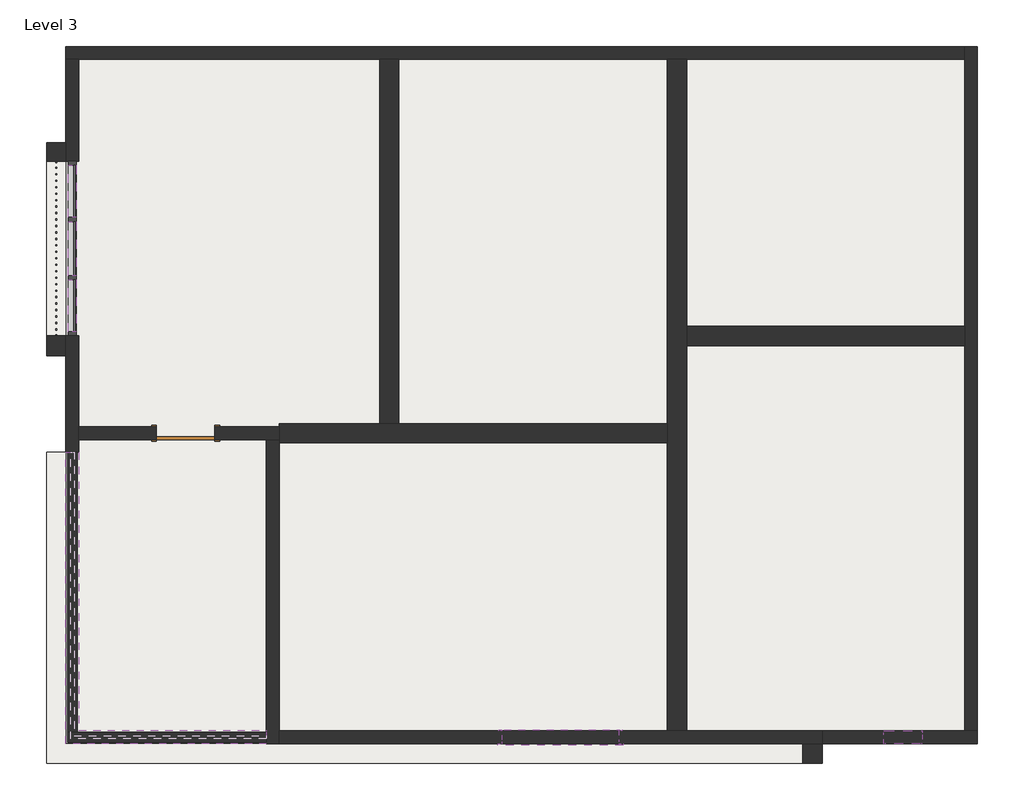
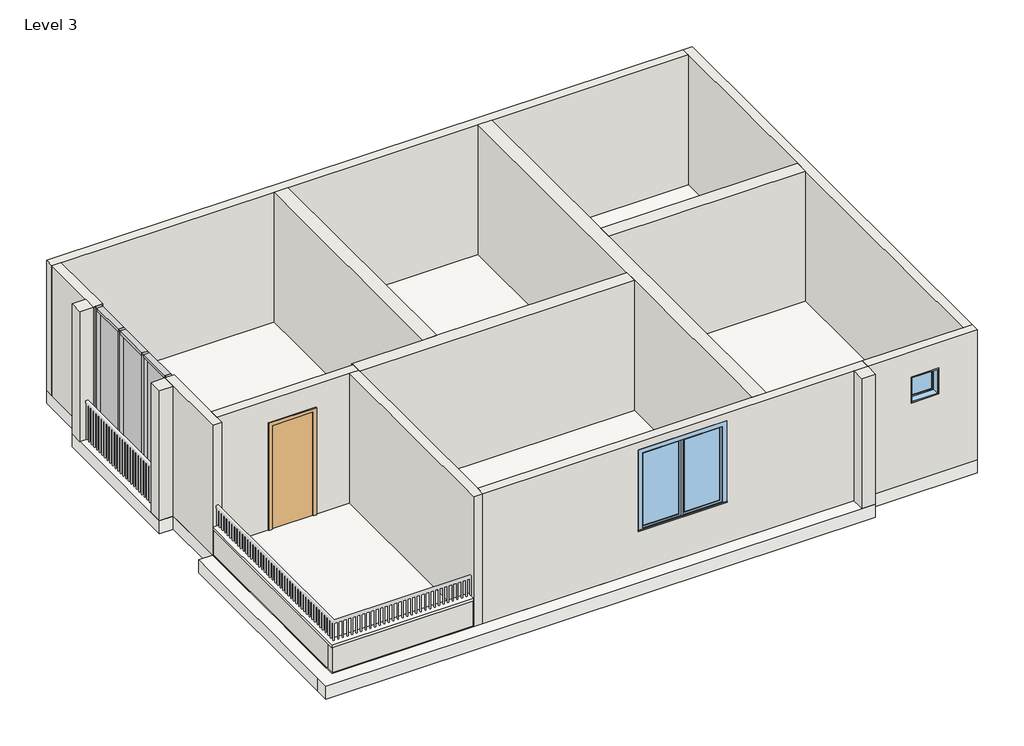
# One storey, part 1 of 2: 17 walls, 10 members, 3 plates, 3 slabs, 2 windows, 1 door.
"""IFC4 building model written with IfcOpenShell, lengths in millimetres."""

from ifc_helpers import new_model, si_unit, frame, origin, place, context, project, spatial, polyline, outline, extrude, faceted_brep, transform, mapped, element, save
from components import door_f936a269, member_eaba9652, member_3f395ae9, member_c17f1be2, member_d2e7e466, system_panel_glazed_52d31088, system_panel_glazed_f0722de2, window_97c6202a, window_6846e476

model = new_model("IFC4")

# Units and contexts
model_context = context("Model", 3, world=origin())
ifc_project = project(units=[si_unit("LENGTHUNIT", "METRE", prefix="MILLI")], contexts=[model_context])

# Site, building, storey
site = spatial("IfcSite", under=ifc_project)
building = spatial("IfcBuilding", under=site)
storey = spatial("IfcBuildingStorey", under=building, Name="Level 3", Elevation=6096.0)

# Door
placement = place(None, origin())
door_shape = door_f936a269(model_context)
element("IfcDoor", 1, ObjectType="Single-Flush : 36\" x 96\"", at=placement, inside=storey, context=model_context, shape_type="MappedRepresentation", body=[
    mapped(door_shape, transform((-16449.2169582, -4610.4617616, 6705.6), x_axis=(-1.0, 0.0, 0.0), y_axis=(0.0, -1.0, 0.0), z_axis=(0.0, 0.0, 1.0))),
])

# Members
member_shape = member_eaba9652(model_context)
element("IfcMember", 2, ObjectType="Rectangular Mullion : 2.5\" x 5\" rectangular", at=placement, inside=storey, context=model_context, shape_type="MappedRepresentation", body=[
    mapped(member_shape, transform((-18227.2169582, -1251.3117616, 6705.6), x_axis=(0.0, -1.0, 0.0), y_axis=(-1.0, 0.0, 0.0), z_axis=(0.0, 0.0, -1.0))),
])
element("IfcMember", 3, ObjectType="Rectangular Mullion : 2.5\" x 5\" rectangular", at=placement, inside=storey, context=model_context, shape_type="MappedRepresentation", body=[
    mapped(member_shape, transform((-18227.2169582, -2165.7117616, 6705.6), x_axis=(0.0, -1.0, 0.0), y_axis=(-1.0, 0.0, 0.0), z_axis=(0.0, 0.0, -1.0))),
])
member_2_shape = member_3f395ae9(model_context)
element("IfcMember", 4, ObjectType="Rectangular Mullion : 2.5\" x 5\" rectangular", at=placement, inside=storey, context=model_context, shape_type="MappedRepresentation", body=[
    mapped(member_2_shape, transform((-18227.2169582, -3080.1117616, 6705.6), x_axis=(0.0, -1.0, 0.0), y_axis=(-1.0, 0.0, 0.0), z_axis=(0.0, 0.0, -1.0))),
])
element("IfcMember", 5, ObjectType="Rectangular Mullion : 2.5\" x 5\" rectangular", at=placement, inside=storey, context=model_context, shape_type="MappedRepresentation", body=[
    mapped(member_2_shape, transform((-18227.2169582, -336.9117616, 9753.6), x_axis=(0.0, 1.0, 0.0), y_axis=(-1.0, 0.0, 0.0), z_axis=(0.0, 0.0, 1.0))),
])
member_3_shape = member_c17f1be2(model_context)
element("IfcMember", 6, ObjectType="Rectangular Mullion : 2.5\" x 5\" rectangular", at=placement, inside=storey, context=model_context, shape_type="MappedRepresentation", body=[
    mapped(member_3_shape, transform((-18227.2169582, -3016.6117616, 9753.6), x_axis=(0.0, 0.0, 1.0), y_axis=(-1.0, 0.0, 0.0), z_axis=(0.0, -1.0, 0.0))),
])
element("IfcMember", 7, ObjectType="Rectangular Mullion : 2.5\" x 5\" rectangular", at=placement, inside=storey, context=model_context, shape_type="MappedRepresentation", body=[
    mapped(member_3_shape, transform((-18227.2169582, -1219.5617616, 9753.6), x_axis=(0.0, 0.0, 1.0), y_axis=(-1.0, 0.0, 0.0), z_axis=(0.0, -1.0, 0.0))),
])
element("IfcMember", 8, ObjectType="Rectangular Mullion : 2.5\" x 5\" rectangular", at=placement, inside=storey, context=model_context, shape_type="MappedRepresentation", body=[
    mapped(member_3_shape, transform((-18227.2169582, -400.4117616, 6705.6), x_axis=(0.0, 0.0, -1.0), y_axis=(-1.0, 0.0, 0.0), z_axis=(0.0, 1.0, 0.0))),
])
element("IfcMember", 9, ObjectType="Rectangular Mullion : 2.5\" x 5\" rectangular", at=placement, inside=storey, context=model_context, shape_type="MappedRepresentation", body=[
    mapped(member_3_shape, transform((-18227.2169582, -2197.4617616, 6705.6), x_axis=(0.0, 0.0, -1.0), y_axis=(-1.0, 0.0, 0.0), z_axis=(0.0, 1.0, 0.0))),
])
member_4_shape = member_d2e7e466(model_context)
element("IfcMember", 10, ObjectType="Rectangular Mullion : 2.5\" x 5\" rectangular", at=placement, inside=storey, context=model_context, shape_type="MappedRepresentation", body=[
    mapped(member_4_shape, transform((-18227.2169582, -1283.0617616, 6705.6), x_axis=(0.0, 0.0, -1.0), y_axis=(-1.0, 0.0, 0.0), z_axis=(0.0, 1.0, 0.0))),
])
element("IfcMember", 11, ObjectType="Rectangular Mullion : 2.5\" x 5\" rectangular", at=placement, inside=storey, context=model_context, shape_type="MappedRepresentation", body=[
    mapped(member_4_shape, transform((-18227.2169582, -2133.9617616, 9753.6), x_axis=(0.0, 0.0, 1.0), y_axis=(-1.0, 0.0, 0.0), z_axis=(0.0, -1.0, 0.0))),
])

# Plates
system_panel_glazed_shape = system_panel_glazed_52d31088(model_context)
element("IfcPlate", 12, ObjectType="System Panel : Glazed", at=placement, inside=storey, context=model_context, shape_type="MappedRepresentation", body=[
    mapped(system_panel_glazed_shape, transform((-18227.2169582, -809.9867616, 6769.1), x_axis=(0.0, -1.0, 0.0), y_axis=(1.0, 0.0, 0.0), z_axis=(0.0, 0.0, 1.0))),
])
element("IfcPlate", 13, ObjectType="System Panel : Glazed", at=placement, inside=storey, context=model_context, shape_type="MappedRepresentation", body=[
    mapped(system_panel_glazed_shape, transform((-18227.2169582, -2607.0367616, 6769.1), x_axis=(0.0, -1.0, 0.0), y_axis=(1.0, 0.0, 0.0), z_axis=(0.0, 0.0, 1.0))),
])
system_panel_glazed_2_shape = system_panel_glazed_f0722de2(model_context)
element("IfcPlate", 14, ObjectType="System Panel : Glazed", at=placement, inside=storey, context=model_context, shape_type="MappedRepresentation", body=[
    mapped(system_panel_glazed_2_shape, transform((-18227.2169582, -1708.5117616, 6769.1), x_axis=(0.0, -1.0, 0.0), y_axis=(1.0, 0.0, 0.0), z_axis=(0.0, 0.0, 1.0))),
])

# Slabs
element("IfcSlab", 15, ObjectType="Generic - 12\"", at=placement, inside=storey, context=model_context, shape_type="SweptSolid", body=[
    extrude(outline(polyline([(-18633.6169582, -41.6299243), (-18328.8169582, -41.6299243), (-18328.8169582, -3394.4299243), (-18633.6169582, -3394.4299243), (-18633.6169582, -41.6299243)])), frame((0.0, 0.0, 6400.8), z_axis=(0.0, 0.0, 1.0), x_axis=(1.0, 0.0, 0.0)), (0.0, 0.0, 1.0), 304.8),
    extrude(outline(polyline([(-18633.6169582, -4908.9117616), (-18328.8169582, -4908.9117616), (-18328.8169582, -9487.2617616), (-6444.7919582, -9487.2617616), (-6444.7919582, -9792.0617616), (-18633.6169582, -9792.0617616), (-18633.6169582, -9487.2617616), (-18633.6169582, -4908.9117616)])), frame((0.0, 0.0, 6400.8), z_axis=(0.0, 0.0, 1.0), x_axis=(1.0, 0.0, 0.0)), (0.0, 0.0, 1.0), 304.8),
])
element("IfcSlab", 16, ObjectType="Generic - 12\" 2", at=placement, inside=storey, context=model_context, shape_type="SweptSolid", body=[
    extrude(outline(polyline([(-4006.3919582, 1466.4882384), (-4006.3919582, -9487.2617616), (-18328.8169582, -9487.2617616), (-18328.8169582, 1466.4882384), (-4006.3919582, 1466.4882384)])), frame((0.0, 0.0, 6400.8), z_axis=(0.0, 0.0, 1.0), x_axis=(1.0, 0.0, 0.0)), (0.0, 0.0, 1.0), 304.8),
])
element("IfcSlab", 17, ObjectType="Generic - 2\"", at=placement, inside=storey, context=model_context, shape_type="SweptSolid", body=[
    extrude(outline(polyline([(-15179.2169582, -9487.2617616), (-18328.8169582, -9487.2617616), (-18328.8169582, -4908.9117616), (-18125.6169582, -4908.9117616), (-18125.6169582, -9277.7117616), (-15179.2169582, -9277.7117616), (-15179.2169582, -9309.4617616), (-15179.2169582, -9487.2617616)])), frame((0.0, 0.0, 7315.2), z_axis=(0.0, 0.0, 1.0), x_axis=(1.0, 0.0, 0.0)), (0.0, 0.0, 1.0), 50.8),
])

# Walls
element("IfcWall", 18, ObjectType="Generic - 12\" white", at=placement, inside=storey, context=model_context, shape_type="SweptSolid", body=[
    extrude(outline(polyline([(-18633.6169582, -336.9117616), (-18633.6169582, -41.6299243), (-18328.8169582, -41.6299243), (-18328.8169582, -336.9117616), (-18633.6169582, -336.9117616)])), frame((0.0, 0.0, 6705.6), z_axis=(0.0, 0.0, 1.0), x_axis=(1.0, 0.0, 0.0)), (0.0, 0.0, 1.0), 3048.0),
])
element("IfcWall", 19, ObjectType="Generic - 12\" white", at=placement, inside=storey, context=model_context, shape_type="SweptSolid", body=[
    extrude(outline(polyline([(-18328.8169582, -3080.1117616), (-18328.8169582, -3394.4299243), (-18633.6169582, -3394.4299243), (-18633.6169582, -3080.1117616), (-18328.8169582, -3080.1117616)])), frame((0.0, 0.0, 6705.6), z_axis=(0.0, 0.0, 1.0), x_axis=(1.0, 0.0, 0.0)), (0.0, 0.0, 1.0), 3048.0),
])
element("IfcWall", 20, ObjectType="Generic - 12\" white", at=placement, inside=storey, context=model_context, shape_type="SweptSolid", body=[
    extrude(outline(polyline([(-6749.5919582, -9487.2617616), (-6444.7919582, -9487.2617616), (-6444.7919582, -9792.0617616), (-6749.5919582, -9792.0617616), (-6749.5919582, -9487.2617616)])), frame((0.0, 0.0, 6705.6), z_axis=(0.0, 0.0, 1.0), x_axis=(1.0, 0.0, 0.0)), (0.0, 0.0, 1.0), 3048.0),
])
element("IfcWall", 21, ObjectType="Generic - 12\" white", at=placement, inside=storey, context=model_context, shape_type="Brep", body=[
    faceted_brep([(-8575.2169582, -9284.0617616, 6705.6), (-8575.2169582, -3232.5117616, 6705.6), (-8575.2169582, -2927.7117616, 6705.6), (-8575.2169582, 1263.2882384, 6705.6), (-8575.2169582, 1263.2882384, 9753.6), (-8575.2169582, -2927.7117616, 9753.6), (-8575.2169582, -3232.5117616, 9753.6), (-8575.2169582, -9284.0617616, 9753.6), (-8880.0169582, -9284.0617616, 6705.6), (-8880.0169582, -9284.0617616, 9753.6), (-8880.0169582, -4762.8617616, 9753.6), (-8880.0169582, -4458.0617616, 9753.6), (-8880.0169582, 1263.2882384, 9753.6), (-8880.0169582, 1263.2882384, 6705.6), (-8880.0169582, -4458.0617616, 6705.6), (-8880.0169582, -4762.8617616, 6705.6)], [[[0, 1, 2, 3, 4, 5, 6, 7]], [[8, 9, 10, 11, 12, 13, 14, 15]], [[3, 2, 1, 0, 8, 15, 14, 13]], [[7, 6, 5, 4, 12, 11, 10, 9]], [[4, 3, 13, 12]], [[0, 7, 9, 8]]]),
])
element("IfcWall", 22, ObjectType="Generic - 12\" white", at=placement, inside=storey, context=model_context, shape_type="Brep", body=[
    faceted_brep([(-14976.0169582, -4762.8617616, 6705.6), (-8880.0169582, -4762.8617616, 6705.6), (-8880.0169582, -4762.8617616, 9753.6), (-14976.0169582, -4762.8617616, 9753.6), (-14976.0169582, -4458.0617616, 6705.6), (-14976.0169582, -4458.0617616, 9753.6), (-13401.2169582, -4458.0617616, 9753.6), (-13096.4169582, -4458.0617616, 9753.6), (-8880.0169582, -4458.0617616, 9753.6), (-8880.0169582, -4458.0617616, 6705.6), (-13096.4169582, -4458.0617616, 6705.6), (-13401.2169582, -4458.0617616, 6705.6), (-14976.0169582, -4712.0617616, 6705.6), (-14976.0169582, -4508.8617616, 6705.6), (-14976.0169582, -4508.8617616, 9753.6), (-14976.0169582, -4712.0617616, 9753.6)], [[[0, 1, 2, 3]], [[4, 5, 6, 7, 8, 9, 10, 11]], [[1, 0, 12, 13, 4, 11, 10, 9]], [[3, 2, 8, 7, 6, 5, 14, 15]], [[0, 3, 15, 14, 5, 4, 13, 12]], [[2, 1, 9, 8]]]),
])
element("IfcWall", 23, ObjectType="Generic - 12\" white", at=placement, inside=storey, context=model_context, shape_type="SweptSolid", body=[
    extrude(outline(polyline([(-13096.4169582, 1263.2882384), (-13096.4169582, -4458.0617616), (-13401.2169582, -4458.0617616), (-13401.2169582, 1263.2882384), (-13096.4169582, 1263.2882384)])), frame((0.0, 0.0, 6705.6), z_axis=(0.0, 0.0, 1.0), x_axis=(1.0, 0.0, 0.0)), (0.0, 0.0, 1.0), 3048.0),
])
element("IfcWall", 24, ObjectType="Generic - 12\" white", at=placement, inside=storey, context=model_context, shape_type="SweptSolid", body=[
    extrude(outline(polyline([(-4209.5919582, -3232.5117616), (-8575.2169582, -3232.5117616), (-8575.2169582, -2927.7117616), (-4209.5919582, -2927.7117616), (-4209.5919582, -3232.5117616)])), frame((0.0, 0.0, 6705.6), z_axis=(0.0, 0.0, 1.0), x_axis=(1.0, 0.0, 0.0)), (0.0, 0.0, 1.0), 3048.0),
])
element("IfcWall", 25, ObjectType="Generic - 6\"", at=placement, inside=storey, context=model_context, shape_type="Brep", body=[
    faceted_brep([(-15179.2169582, -9309.4617616, 6705.6), (-18151.0169582, -9309.4617616, 6705.6), (-18303.4169582, -9309.4617616, 6705.6), (-18303.4169582, -9309.4617616, 7315.2), (-18151.0169582, -9309.4617616, 7315.2), (-15179.2169582, -9309.4617616, 7315.2), (-15179.2169582, -9461.8617616, 6705.6), (-15179.2169582, -9461.8617616, 7315.2), (-18303.4169582, -9461.8617616, 7315.2), (-18303.4169582, -9461.8617616, 6705.6)], [[[0, 1, 2, 3, 4, 5]], [[6, 7, 8, 9]], [[2, 1, 0, 6, 9]], [[5, 4, 3, 8, 7]], [[0, 5, 7, 6]], [[3, 2, 9, 8]]]),
])
element("IfcWall", 26, ObjectType="Generic - 6\"", at=placement, inside=storey, context=model_context, shape_type="SweptSolid", body=[
    extrude(outline(polyline([(-18151.0169582, -4908.9117616), (-18151.0169582, -9309.4617616), (-18303.4169582, -9309.4617616), (-18303.4169582, -4908.9117616), (-18151.0169582, -4908.9117616)])), frame((0.0, 0.0, 6705.6), z_axis=(0.0, 0.0, 1.0), x_axis=(1.0, 0.0, 0.0)), (0.0, 0.0, 1.0), 609.6),
])
element("IfcWall", 27, ObjectType="Generic - 8\"", at=placement, inside=storey, context=model_context, shape_type="Brep", body=[
    faceted_brep([(-4006.3919582, -9284.0617616, 6705.6), (-4006.3919582, 1466.4882384, 6705.6), (-4006.3919582, 1466.4882384, 9753.6), (-4006.3919582, -9284.0617616, 9753.6), (-4209.5919582, -9284.0617616, 6705.6), (-4209.5919582, -9284.0617616, 9753.6), (-4209.5919582, -3232.5117616, 9753.6), (-4209.5919582, -2927.7117616, 9753.6), (-4209.5919582, 1263.2882384, 9753.6), (-4209.5919582, 1466.4882384, 9753.6), (-4209.5919582, 1466.4882384, 6705.6), (-4209.5919582, 1263.2882384, 6705.6), (-4209.5919582, -2927.7117616, 6705.6), (-4209.5919582, -3232.5117616, 6705.6)], [[[0, 1, 2, 3]], [[4, 5, 6, 7, 8, 9, 10, 11, 12, 13]], [[1, 0, 4, 13, 12, 11, 10]], [[3, 2, 9, 8, 7, 6, 5]], [[0, 3, 5, 4]], [[2, 1, 10, 9]]]),
])
element("IfcWall", 28, ObjectType="Generic - 8\"", at=placement, inside=storey, context=model_context, shape_type="Brep", body=[
    faceted_brep([(-4209.5919582, 1466.4882384, 6705.6), (-18328.8169582, 1466.4882384, 6705.6), (-18328.8169582, 1466.4882384, 9753.6), (-4209.5919582, 1466.4882384, 9753.6), (-4209.5919582, 1263.2882384, 6705.6), (-4209.5919582, 1263.2882384, 9753.6), (-8575.2169582, 1263.2882384, 9753.6), (-8880.0169582, 1263.2882384, 9753.6), (-13096.4169582, 1263.2882384, 9753.6), (-13401.2169582, 1263.2882384, 9753.6), (-18125.6169582, 1263.2882384, 9753.6), (-18328.8169582, 1263.2882384, 9753.6), (-18328.8169582, 1263.2882384, 6705.6), (-18125.6169582, 1263.2882384, 6705.6), (-13401.2169582, 1263.2882384, 6705.6), (-13096.4169582, 1263.2882384, 6705.6), (-8880.0169582, 1263.2882384, 6705.6), (-8575.2169582, 1263.2882384, 6705.6)], [[[0, 1, 2, 3]], [[4, 5, 6, 7, 8, 9, 10, 11, 12, 13, 14, 15, 16, 17]], [[1, 0, 4, 17, 16, 15, 14, 13, 12]], [[3, 2, 11, 10, 9, 8, 7, 6, 5]], [[0, 3, 5, 4]], [[2, 1, 12, 11]]]),
])
element("IfcWall", 29, ObjectType="Generic - 8\"", at=placement, inside=storey, context=model_context, shape_type="SweptSolid", body=[
    extrude(outline(polyline([(-18328.8169582, -336.9117616), (-18328.8169582, 1263.2882384), (-18125.6169582, 1263.2882384), (-18125.6169582, -336.9117616), (-18328.8169582, -336.9117616)])), frame((0.0, 0.0, 6705.6), z_axis=(0.0, 0.0, 1.0), x_axis=(1.0, 0.0, 0.0)), (0.0, 0.0, 1.0), 3048.0),
])
element("IfcWall", 30, ObjectType="Generic - 8\"", at=placement, inside=storey, context=model_context, shape_type="Brep", body=[
    faceted_brep([(-18328.8169582, -3080.1117616, 6705.6), (-18328.8169582, -4908.9117616, 6705.6), (-18328.8169582, -4908.9117616, 9753.6), (-18328.8169582, -3080.1117616, 9753.6), (-18125.6169582, -3080.1117616, 6705.6), (-18125.6169582, -3080.1117616, 9753.6), (-18125.6169582, -4508.8617616, 9753.6), (-18125.6169582, -4712.0617616, 9753.6), (-18125.6169582, -4908.9117616, 9753.6), (-18125.6169582, -4908.9117616, 6705.6), (-18125.6169582, -4712.0617616, 6705.6), (-18125.6169582, -4508.8617616, 6705.6), (-18151.0169582, -4908.9117616, 6705.6), (-18303.4169582, -4908.9117616, 6705.6)], [[[0, 1, 2, 3]], [[4, 5, 6, 7, 8, 9, 10, 11]], [[1, 0, 4, 11, 10, 9, 12, 13]], [[2, 1, 13, 12, 9, 8]], [[3, 2, 8, 7, 6, 5]], [[0, 3, 5, 4]]]),
])
element("IfcWall", 31, ObjectType="Generic - 8\" 2", at=placement, inside=storey, context=model_context, shape_type="Brep", body=[
    faceted_brep([(-4006.3919582, -9284.0617616, 6705.6), (-4209.5919582, -9284.0617616, 6705.6), (-6444.7919582, -9284.0617616, 6705.6), (-6444.7919582, -9284.0617616, 9753.6), (-4209.5919582, -9284.0617616, 9753.6), (-4006.3919582, -9284.0617616, 9753.6), (-4869.9919582, -9284.0617616, 9161.8087386), (-5479.5919582, -9284.0617616, 9161.8087386), (-5479.5919582, -9284.0617616, 8552.2087386), (-4869.9919582, -9284.0617616, 8552.2087386), (-4006.3919582, -9487.2617616, 6705.6), (-4006.3919582, -9487.2617616, 9753.6), (-6444.7919582, -9487.2617616, 9753.6), (-6444.7919582, -9487.2617616, 6705.6), (-4869.9919582, -9487.2617616, 9161.8087386), (-4869.9919582, -9487.2617616, 8552.2087386), (-5479.5919582, -9487.2617616, 8552.2087386), (-5479.5919582, -9487.2617616, 9161.8087386)], [[[0, 1, 2, 3, 4, 5], [6, 7, 8, 9]], [[10, 11, 12, 13], [14, 15, 16, 17]], [[2, 1, 0, 10, 13]], [[3, 2, 13, 12]], [[5, 4, 3, 12, 11]], [[0, 5, 11, 10]], [[15, 14, 6, 9]], [[16, 15, 9, 8]], [[17, 16, 8, 7]], [[14, 17, 7, 6]]]),
])
element("IfcWall", 32, ObjectType="Generic - 8\" 3", at=placement, inside=storey, context=model_context, shape_type="Brep", body=[
    faceted_brep([(-14976.0169582, -4712.0617616, 9753.6), (-15179.2169582, -4712.0617616, 9753.6), (-18125.6169582, -4712.0617616, 9753.6), (-18125.6169582, -4712.0617616, 6705.6), (-16906.4169582, -4712.0617616, 6705.6), (-16906.4169582, -4712.0617616, 9144.0), (-15992.0169582, -4712.0617616, 9144.0), (-15992.0169582, -4712.0617616, 6705.6), (-15179.2169582, -4712.0617616, 6705.6), (-14976.0169582, -4712.0617616, 6705.6), (-18125.6169582, -4508.8617616, 9753.6), (-14976.0169582, -4508.8617616, 9753.6), (-14976.0169582, -4508.8617616, 6705.6), (-15992.0169582, -4508.8617616, 6705.6), (-15992.0169582, -4508.8617616, 9144.0), (-16906.4169582, -4508.8617616, 9144.0), (-16906.4169582, -4508.8617616, 6705.6), (-18125.6169582, -4508.8617616, 6705.6)], [[[0, 1, 2, 3, 4, 5, 6, 7, 8, 9]], [[10, 11, 12, 13, 14, 15, 16, 17]], [[3, 17, 16, 4]], [[12, 9, 8, 7, 13]], [[2, 1, 0, 11, 10]], [[3, 2, 10, 17]], [[0, 9, 12, 11]], [[15, 5, 4, 16]], [[5, 15, 14, 6]], [[6, 14, 13, 7]]]),
])
element("IfcWall", 33, ObjectType="Generic - 8\" 3", at=placement, inside=storey, context=model_context, shape_type="Brep", body=[
    faceted_brep([(-15179.2169582, -4712.0617616, 6705.6), (-15179.2169582, -9309.4617616, 6705.6), (-15179.2169582, -9461.8617616, 6705.6), (-15179.2169582, -9487.2617616, 6705.6), (-15179.2169582, -9487.2617616, 9753.6), (-15179.2169582, -4712.0617616, 9753.6), (-14976.0169582, -4712.0617616, 6705.6), (-14976.0169582, -4712.0617616, 9753.6), (-14976.0169582, -4762.8617616, 9753.6), (-14976.0169582, -9284.0617616, 9753.6), (-14976.0169582, -9487.2617616, 9753.6), (-14976.0169582, -9487.2617616, 6705.6), (-14976.0169582, -9284.0617616, 6705.6), (-14976.0169582, -4762.8617616, 6705.6)], [[[0, 1, 2, 3, 4, 5]], [[6, 7, 8, 9, 10, 11, 12, 13]], [[3, 2, 1, 0, 6, 13, 12, 11]], [[5, 4, 10, 9, 8, 7]], [[0, 5, 7, 6]], [[3, 11, 10, 4]]]),
])
element("IfcWall", 34, ObjectType="Generic - 8\" 3", at=placement, inside=storey, context=model_context, shape_type="Brep", body=[
    faceted_brep([(-6444.7919582, -9284.0617616, 6705.6), (-8575.2169582, -9284.0617616, 6705.6), (-8880.0169582, -9284.0617616, 6705.6), (-14976.0169582, -9284.0617616, 6705.6), (-14976.0169582, -9284.0617616, 9753.6), (-8880.0169582, -9284.0617616, 9753.6), (-8575.2169582, -9284.0617616, 9753.6), (-6444.7919582, -9284.0617616, 9753.6), (-11470.8169582, -9284.0617616, 9503.8375963), (-11470.8169582, -9284.0617616, 7675.0375963), (-9642.0169582, -9284.0617616, 7675.0375963), (-9642.0169582, -9284.0617616, 9503.8375963), (-6444.7919582, -9487.2617616, 6705.6), (-6444.7919582, -9487.2617616, 9753.6), (-14976.0169582, -9487.2617616, 9753.6), (-14976.0169582, -9487.2617616, 6705.6), (-11470.8169582, -9487.2617616, 9503.8375963), (-9642.0169582, -9487.2617616, 9503.8375963), (-9642.0169582, -9487.2617616, 7675.0375963), (-11470.8169582, -9487.2617616, 7675.0375963)], [[[0, 1, 2, 3, 4, 5, 6, 7], [8, 9, 10, 11]], [[12, 13, 14, 15], [16, 17, 18, 19]], [[3, 2, 1, 0, 12, 15]], [[7, 6, 5, 4, 14, 13]], [[0, 7, 13, 12]], [[3, 15, 14, 4]], [[9, 8, 16, 19]], [[10, 9, 19, 18]], [[11, 10, 18, 17]], [[8, 11, 17, 16]]]),
])

# Windows
window_shape = window_97c6202a(model_context)
element("IfcWindow", 35, ObjectType="Casement Dbl with Trim.0001 : 72\" x 72\"", at=placement, inside=storey, context=model_context, shape_type="MappedRepresentation", body=[
    mapped(window_shape, transform((-10556.4169582, -9366.6117616, 6760.6375963), x_axis=(-1.0, 0.0, 0.0), y_axis=(0.0, -1.0, 0.0), z_axis=(0.0, 0.0, 1.0))),
])
window_2_shape = window_6846e476(model_context)
element("IfcWindow", 36, ObjectType="Fixed : 24\" x 24\"", at=placement, inside=storey, context=model_context, shape_type="MappedRepresentation", body=[
    mapped(window_2_shape, transform((-5136.6919582, -9385.6617616, 7637.8087386), x_axis=(1.0, 0.0, 0.0), y_axis=(0.0, 1.0, 0.0), z_axis=(0.0, 0.0, 1.0))),
])

save(model, "model.ifc")

# Revit data of these elements
# Type "Single-Flush : 36\" x 96\""
#   Type Mark = "1"
#   Construction Type Id = "MDOOR"
#   Assembly Code = "C1020"
#   Analytic Construction = "Metal"
#   Thickness = 0' - 2"
#   Heat Transfer Coefficient (U) = 0.651978 BTU/(h·ft²·°F)
#   Height = 8' - 0"
#   Trim Projection Ext = 0' - 1"
#   Trim Projection Int = 0' - 1"
#   Trim Width = 0' - 3"
#   Width = 3' - 0"
#   Define Thermal Properties by = 1
#   Door Material = Glass, Clear Glazing
#   Frame Material = Iron, Ductile
#   Visual Light Transmittance = 0
#   Solar Heat Gain Coefficient = 0
#   Function = (empty or 0)
#   Wall Closure = (empty or 0)
# Type "Rectangular Mullion : 2.5\" x 5\" rectangular"
#   built-in parameter 1007304 = 0.416667 (stored number, unit not read)
#   built-in parameter 1007301 = 0.104167 (stored number, unit not read)
#   built-in parameter 1007300 = 0.104167 (stored number, unit not read)
# Type "System Panel : Glazed"
#   Construction Type Id = "GSP4R"
#   Analytic Construction = "1/8 in Pilkington single glazing"
#   Visual Light Transmittance = 0.9
#   Solar Heat Gain Coefficient = 0.86
#   Heat Transfer Coefficient (U) = 1.18115 BTU/(h·ft²·°F)
# Type "Generic - 12\""
#   Assembly Code = "B1010"
#   Function = 0
#   Layers, outside or top first: 1' - 0" "Parking Stripe" (function 1)
# Type "Generic - 12\" 2"
#   Assembly Code = "B1010"
#   Function = 0
#   Layers, outside or top first: 1' - 0" "Parking Stripe" (function 1)
# Type "Generic - 2\""
#   Assembly Code = "B1010"
#   Function = 0
#   Layers, outside or top first: 0' - 2" "Parking Stripe" (function 1)
# Type "Generic - 12\" white"
#   Assembly Code = "B2010"
#   Layers, outside or top first: 1' - 0" "Parking Stripe" (function 1)
# Type "Generic - 6\""
#   Assembly Code = "B2010"
#   Layers, outside or top first: 0' - 6" "Concrete Masonry Units" (function 1)
# Type "Generic - 8\""
#   Assembly Code = "B2010"
#   Layers, outside or top first: 0' - 8" "Door - Frame" (function 1)
# Type "Generic - 8\" 2"
#   Assembly Code = "B2010"
#   Layers, outside or top first: 0' - 8" "Door - Frame" (function 1)
# Type "Generic - 8\" 3"
#   Assembly Code = "B2010"
#   Layers, outside or top first: 0' - 8" "EIFS, Exterior Insulation" (function 1)
# Type "Casement Dbl with Trim.0001 : 72\" x 72\""
#   Type Mark = "10"
#   Construction Type Id = "GSP4R"
#   Assembly Code = "B2020100"
#   Analytic Construction = "1/8 in Pilkington single glazing"
#   Visual Light Transmittance = 0.9
#   Solar Heat Gain Coefficient = 0.78
#   Heat Transfer Coefficient (U) = 0.6496 BTU/(h·ft²·°F)
#   Height = 6' - 0"
#   Default Sill Height = 3' - 0"
#   Trim Projection - Ext. = 0' - 0 1/2"
#   Trim Projection - Int. = 0' - 0 3/4"
#   Trim Width - Exterior = 0' - 3 1/2"
#   Trim Width - Interior = 0' - 3 1/2"
#   Width = 6' - 0"
#   Window Inset = 0' - 0 3/4"
#   Define Thermal Properties by = 1
#   Glass Pane Material = Glass
#   Sash Material = Iron, Ductile
#   Trim Exterior Material = Iron, Ductile
#   Trim Interior Material = Iron, Ductile
#   Wall Closure = (empty or 0)
# Type "Fixed : 24\" x 24\""
#   Type Mark = "3"
#   Construction Type Id = "GSP4R"
#   Assembly Code = "B2020100"
#   Analytic Construction = "1/8 in Pilkington single glazing"
#   Visual Light Transmittance = 0.9
#   Solar Heat Gain Coefficient = 0.78
#   Heat Transfer Coefficient (U) = 0.6496 BTU/(h·ft²·°F)
#   Height = 2' - 0"
#   Default Sill Height = 3' - 0"
#   Width = 2' - 0"
#   Window Inset = 0' - 0 3/4"
#   Define Thermal Properties by = 1
#   Glass Pane Material = Glass
#   Sash Material = Iron, Ductile
#   Wall Closure = (empty or 0)
# Element 1 (IfcDoor, "Single-Flush : 36\" x 96\"")
#   Phase Created = New Construction
#   Materials on its faces: "Iron, Ductile", "Glass, Clear Glazing"
# Elements 2, 3, 4, 5, 6, 7, 8, 9, 10, 11 (IfcMember, "Rectangular Mullion : 2.5\" x 5\" rectangular")
#   Phase Created = New Construction
#   Materials on its faces: "Iron, Ductile"
# Elements 12, 13, 14 (IfcPlate, "System Panel : Glazed")
#   Phase Created = New Construction
#   Materials on its faces: "Glass"
# Element 15 (IfcSlab, "Generic - 12\"")
#   built-in parameter 1001955 = 3.14159 (stored number, unit not read)
#   Height Offset From Level = 2' - 0"
#   Phase Created = New Construction
#   Materials on its faces: "Parking Stripe"
# Element 16 (IfcSlab, "Generic - 12\" 2")
#   Height Offset From Level = 2' - 0"
#   Phase Created = New Construction
#   Materials on its faces: "Parking Stripe"
# Element 17 (IfcSlab, "Generic - 2\"")
#   built-in parameter 1001955 = -1.5708 (stored number, unit not read)
#   Height Offset From Level = 4' - 2"
#   Phase Created = New Construction
#   Materials on its faces: "Parking Stripe"
# Elements 18, 19, 20, 21, 22, 23, 24 (IfcWall, "Generic - 12\" white")
#   built-in parameter 1001111 = 2' - 0"
#   Top Offset = 0' - 0"
#   Base Offset = 2' - 0"
#   Unconnected Height = 10' - 0"
#   wall height = 10' - 0"
#   Phase Created = New Construction
#   Base Constraint = Level 3
#   Materials on its faces: "Parking Stripe"
# Elements 25, 26 (IfcWall, "Generic - 6\"")
#   built-in parameter 1001111 = 2' - 0"
#   Top Offset = 0' - 0"
#   Base Offset = 2' - 0"
#   Unconnected Height = 2' - 0"
#   wall height = 2' - 0"
#   Phase Created = New Construction
#   Base Constraint = Level 3
#   Materials on its faces: "Concrete Masonry Units"
# Elements 27, 28, 29, 30 (IfcWall, "Generic - 8\"")
#   built-in parameter 1001111 = 2' - 0"
#   Top Offset = 0' - 0"
#   Base Offset = 2' - 0"
#   Unconnected Height = 10' - 0"
#   wall height = 10' - 0"
#   Phase Created = New Construction
#   Base Constraint = Level 3
#   Materials on its faces: "Door - Frame"
# Element 31 (IfcWall, "Generic - 8\" 2")
#   built-in parameter 1001111 = 2' - 0"
#   Top Offset = 0' - 0"
#   Base Offset = 2' - 0"
#   Unconnected Height = 10' - 0"
#   wall height = 10' - 0"
#   Phase Created = New Construction
#   Base Constraint = Level 3
#   Materials on its faces: "Door - Frame"
# Elements 32, 33, 34 (IfcWall, "Generic - 8\" 3")
#   built-in parameter 1001111 = 2' - 0"
#   Top Offset = 0' - 0"
#   Base Offset = 2' - 0"
#   Unconnected Height = 10' - 0"
#   wall height = 10' - 0"
#   Phase Created = New Construction
#   Base Constraint = Level 3
#   Materials on its faces: "EIFS, Exterior Insulation"
# Element 35 (IfcWindow, "Casement Dbl with Trim.0001 : 72\" x 72\"")
#   Mark = "4"
#   Phase Created = New Construction
#   Materials on its faces: "Iron, Ductile", "Glass"
# Element 36 (IfcWindow, "Fixed : 24\" x 24\"")
#   Mark = "3"
#   Phase Created = New Construction
#   Materials on its faces: "Iron, Ductile", "Glass"
# Materials
#   "Glass, Clear Glazing": class "Glass", colour RGB 0 128 192, transparency 0.75, Description = "Clear glazing", Cost = 0
#   "Iron, Ductile": class "Metal", colour RGB 0 0 0, transparency 0, Description = "Ductile cast iron", Cost = 0
#   "Parking Stripe": class "Paint", colour RGB 250 250 91, transparency 0, Cost = 0
#   "Concrete Masonry Units": class "Masonry", colour RGB 227 227 227, transparency 0, Description = "Concrete masonry units", Cost = 0
#   "Door - Frame": colour RGB 118 70 51, transparency 0, Cost = 0
#   "EIFS, Exterior Insulation": class "Generic", colour RGB 127 127 127, transparency 0, Description = "EIFS - Exterior Insulation", Cost = 0
#   "Glass": class "Glass", colour RGB 0 128 192, transparency 0.75, Description = "Soda Lime Glass", Cost = 0
